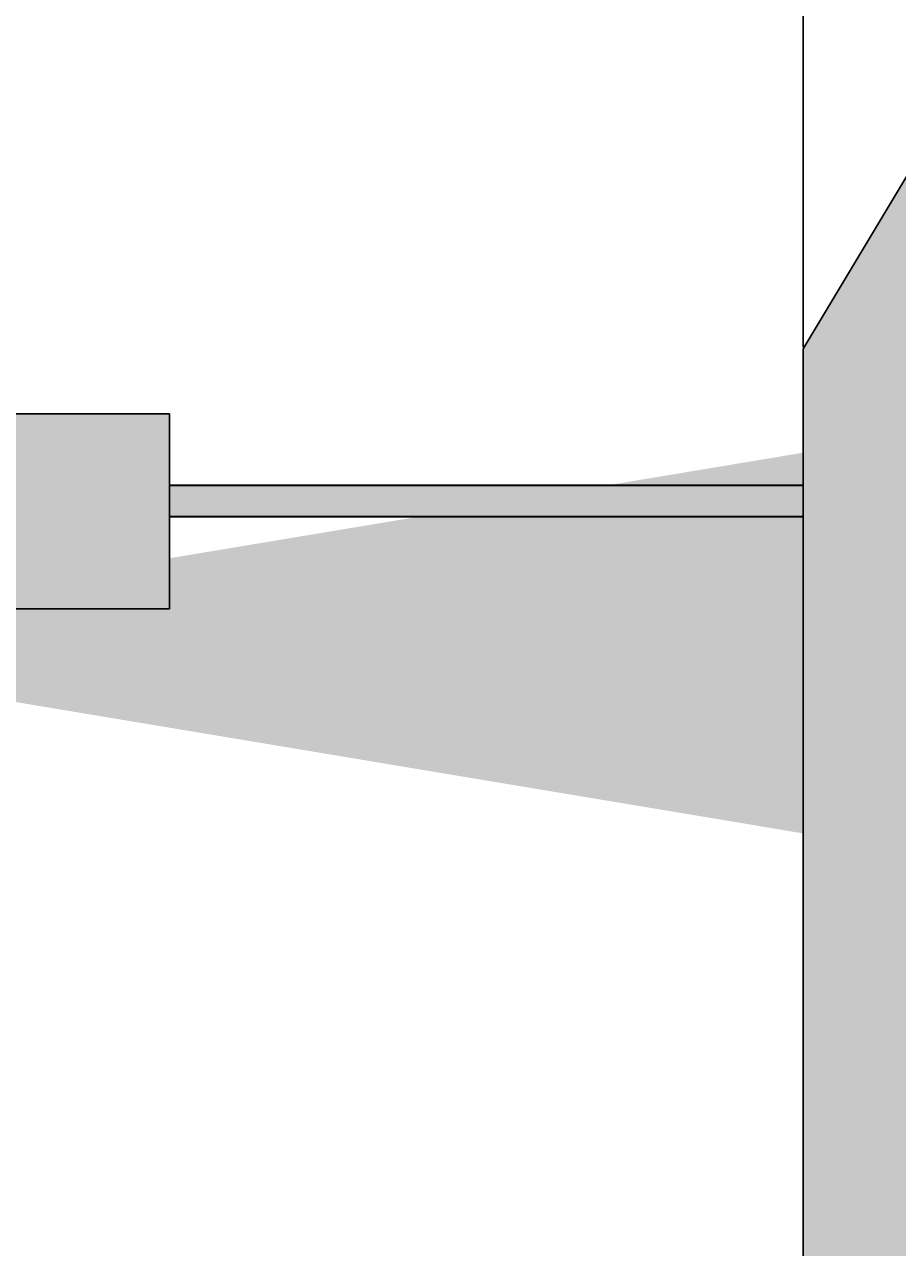
# Model space of a CAD drawing. Units: millimetres. Extents: x -22994 to 29398, y -19990 to 20176.
# Tile 24 of 135: x 71 to 99, y 99 to 138. Entities that reach past the tile are written whole.
import ezdxf

# ---------------------------------------------------------------- set-up
doc = ezdxf.new("R2010")
doc.units = ezdxf.units.MM
doc.header["$MEASUREMENT"] = 0
for name, color, linetype, lineweight in [('M-DIMS', 2, 'Continuous', 18), ('M-EQPM', 7, 'Continuous', 25), ('M-EQPM-PATT', 7, 'Continuous', 18), ('M-PIPE', 7, 'Continuous', 35)]:
    doc.layers.add(name, color=color, linetype=linetype, lineweight=lineweight)
doc.styles.get("Standard").update_dxf_attribs({"font": 'arial.ttf'})
doc.dimstyles.get("Standard").update_dxf_attribs({"dimtxt": 0.18, "dimasz": 10000, "dimexe": 0.18, "dimexo": 0.0625, "dimgap": 0.09, "dimtad": 0, "dimtih": 1, "dimtoh": 1, "dimdec": 0, "dimzin": 0, "dimdsep": 46, "dimtxsty": 'Standard', "dimcen": 0.09, "dimadec": 0, "dimazin": 0, "dimtfac": 1, "dimtdec": 0, "dimtofl": 0, "dimtmove": 0, "dimatfit": 3, "dimfxl": 1, "dimtolj": 1, "dimtzin": 0, "dimlwd": 30, "dimarcsym": 0})

# ---------------------------------------------------------------- blocks, each defined once
blk = doc.blocks.new('*D2')
at = {"layer": 'Defpoints', "color": 0, "transparency": 16777216}
for p in [(6.677, 10.271), (290.852, 10.271), (290.852, -5.079)]:
    blk.add_point(p, dxfattribs=at)
at = {"layer": 'M-DIMS', "color": 0, "lineweight": -2, "transparency": 16777216}
for p, q in [((6.677, 10.209), (6.677, -5.259)), ((290.852, 10.209), (290.852, -5.259))]:
    blk.add_line(p, q, dxfattribs=at)
at = {"layer": 'M-DIMS', "color": 0, "lineweight": 30, "transparency": 16777216}
for p, q in [((-9993.323, -5.079), (-19993.323, -5.079)), ((10290.852, -5.079), (20290.852, -5.079))]:
    blk.add_line(p, q, dxfattribs=at)
at = {"layer": 'M-DIMS', "color": 0, "transparency": 16777216}
for points in [[(-9993.323, 1661.588), (-9993.323, -1671.745), (6.677, -5.079)], [(10290.852, 1661.588), (10290.852, -1671.745), (290.852, -5.079)]]:
    blk.add_solid(points, dxfattribs=at)
at = {"layer": 'M-DIMS', "color": 0, "transparency": 16777216, "insert": (148.765, -5.079), "char_height": 0.18, "attachment_point": 5}
blk.add_mtext('\\A1;284.2', dxfattribs=at)
blk = doc.blocks.new('*D3')
at = {"layer": 'Defpoints', "color": 0, "transparency": 16777216}
for p in [(110.265, 204.165), (110.265, 176.366), (95.833, 127.967)]:
    blk.add_point(p, dxfattribs=at)
at = {"layer": 'M-DIMS', "color": 0, "lineweight": -2, "transparency": 16777216}
for p, q in [((95.833, 128.03), (95.833, 204.345)), ((110.265, 176.429), (110.265, 204.345))]:
    blk.add_line(p, q, dxfattribs=at)
at = {"layer": 'M-DIMS', "color": 0, "lineweight": 30, "transparency": 16777216}
for p, q in [((-9904.167, 204.165), (-19904.167, 204.165)), ((10110.265, 204.165), (20110.265, 204.165))]:
    blk.add_line(p, q, dxfattribs=at)
at = {"layer": 'M-DIMS', "color": 0, "transparency": 16777216}
for points in [[(-9904.167, 1870.832), (-9904.167, -1462.501), (95.833, 204.165)], [(10110.265, 1870.832), (10110.265, -1462.501), (110.265, 204.165)]]:
    blk.add_solid(points, dxfattribs=at)
at = {"layer": 'M-DIMS', "color": 0, "transparency": 16777216, "insert": (103.049, 204.165), "char_height": 0.18, "attachment_point": 5}
blk.add_mtext('\\A1;14.432', dxfattribs=at)
blk = doc.blocks.new('*D4')
at = {"layer": 'Defpoints', "color": 0, "transparency": 16777216}
for p in [(116.265, 204.165), (110.265, 176.366), (116.265, 176.366)]:
    blk.add_point(p, dxfattribs=at)
at = {"layer": 'M-DIMS', "color": 0, "lineweight": -2, "transparency": 16777216}
for p, q in [((110.265, 176.429), (110.265, 204.345)), ((116.265, 176.429), (116.265, 204.345))]:
    blk.add_line(p, q, dxfattribs=at)
at = {"layer": 'M-DIMS', "color": 0, "lineweight": 30, "transparency": 16777216}
for p, q in [((-9889.735, 204.165), (-19889.735, 204.165)), ((10116.265, 204.165), (20116.265, 204.165))]:
    blk.add_line(p, q, dxfattribs=at)
at = {"layer": 'M-DIMS', "color": 0, "transparency": 16777216}
for points in [[(-9889.735, 1870.832), (-9889.735, -1462.501), (110.265, 204.165)], [(10116.265, 1870.832), (10116.265, -1462.501), (116.265, 204.165)]]:
    blk.add_solid(points, dxfattribs=at)
at = {"layer": 'M-DIMS', "color": 0, "transparency": 16777216, "insert": (113.265, 204.165), "char_height": 0.18, "attachment_point": 5}
blk.add_mtext('\\A1;6', dxfattribs=at)
blk = doc.blocks.new('*D5')
at = {"layer": 'Defpoints', "color": 0, "transparency": 16777216}
for p in [(181.265, 204.165), (116.265, 176.366), (181.265, 176.366)]:
    blk.add_point(p, dxfattribs=at)
at = {"layer": 'M-DIMS', "color": 0, "lineweight": -2, "transparency": 16777216}
for p, q in [((116.265, 176.429), (116.265, 204.345)), ((181.265, 176.429), (181.265, 204.345))]:
    blk.add_line(p, q, dxfattribs=at)
at = {"layer": 'M-DIMS', "color": 0, "lineweight": 30, "transparency": 16777216}
for p, q in [((-9883.735, 204.165), (-19883.735, 204.165)), ((10181.265, 204.165), (20181.265, 204.165))]:
    blk.add_line(p, q, dxfattribs=at)
at = {"layer": 'M-DIMS', "color": 0, "transparency": 16777216}
for points in [[(-9883.735, 1870.832), (-9883.735, -1462.501), (116.265, 204.165)], [(10181.265, 1870.832), (10181.265, -1462.501), (181.265, 204.165)]]:
    blk.add_solid(points, dxfattribs=at)
at = {"layer": 'M-DIMS', "color": 0, "transparency": 16777216, "insert": (148.765, 204.165), "char_height": 0.18, "attachment_point": 5}
blk.add_mtext('\\A1;65', dxfattribs=at)
blk = doc.blocks.new('*D6')
at = {"layer": 'Defpoints', "color": 0, "transparency": 16777216}
for p in [(187.265, 204.165), (181.265, 176.366), (187.265, 176.366)]:
    blk.add_point(p, dxfattribs=at)
at = {"layer": 'M-DIMS', "color": 0, "lineweight": -2, "transparency": 16777216}
for p, q in [((181.265, 176.429), (181.265, 204.345)), ((187.265, 176.429), (187.265, 204.345))]:
    blk.add_line(p, q, dxfattribs=at)
at = {"layer": 'M-DIMS', "color": 0, "lineweight": 30, "transparency": 16777216}
for p, q in [((-9818.735, 204.165), (-19818.735, 204.165)), ((10187.265, 204.165), (20187.265, 204.165))]:
    blk.add_line(p, q, dxfattribs=at)
at = {"layer": 'M-DIMS', "color": 0, "transparency": 16777216}
for points in [[(-9818.735, 1870.832), (-9818.735, -1462.501), (181.265, 204.165)], [(10187.265, 1870.832), (10187.265, -1462.501), (187.265, 204.165)]]:
    blk.add_solid(points, dxfattribs=at)
at = {"layer": 'M-DIMS', "color": 0, "transparency": 16777216, "insert": (184.265, 204.165), "char_height": 0.18, "attachment_point": 5}
blk.add_mtext('\\A1;6', dxfattribs=at)
blk = doc.blocks.new('*D7')
at = {"layer": 'Defpoints', "color": 0, "transparency": 16777216}
for p in [(201.697, 204.165), (187.265, 176.366), (201.697, 127.967)]:
    blk.add_point(p, dxfattribs=at)
at = {"layer": 'M-DIMS', "color": 0, "lineweight": -2, "transparency": 16777216}
for p, q in [((187.265, 176.429), (187.265, 204.345)), ((201.697, 128.03), (201.697, 204.345))]:
    blk.add_line(p, q, dxfattribs=at)
at = {"layer": 'M-DIMS', "color": 0, "lineweight": 30, "transparency": 16777216}
for p, q in [((-9812.735, 204.165), (-19812.735, 204.165)), ((10201.697, 204.165), (20201.697, 204.165))]:
    blk.add_line(p, q, dxfattribs=at)
at = {"layer": 'M-DIMS', "color": 0, "transparency": 16777216}
for points in [[(-9812.735, 1870.832), (-9812.735, -1462.501), (187.265, 204.165)], [(10201.697, 1870.832), (10201.697, -1462.501), (201.697, 204.165)]]:
    blk.add_solid(points, dxfattribs=at)
at = {"layer": 'M-DIMS', "color": 0, "transparency": 16777216, "insert": (194.481, 204.165), "char_height": 0.18, "attachment_point": 5}
blk.add_mtext('\\A1;14.432', dxfattribs=at)
blk = doc.blocks.new('*D8')
at = {"layer": 'Defpoints', "color": 0, "transparency": 16777216}
for p in [(227.648, 204.165), (227.648, 146.73), (201.697, 127.967)]:
    blk.add_point(p, dxfattribs=at)
at = {"layer": 'M-DIMS', "color": 0, "lineweight": -2, "transparency": 16777216}
for p, q in [((201.697, 128.03), (201.697, 204.345)), ((227.648, 146.792), (227.648, 204.345))]:
    blk.add_line(p, q, dxfattribs=at)
at = {"layer": 'M-DIMS', "color": 0, "lineweight": 30, "transparency": 16777216}
for p, q in [((-9798.303, 204.165), (-19798.303, 204.165)), ((10227.648, 204.165), (20227.648, 204.165))]:
    blk.add_line(p, q, dxfattribs=at)
at = {"layer": 'M-DIMS', "color": 0, "transparency": 16777216}
for points in [[(-9798.303, 1870.832), (-9798.303, -1462.501), (201.697, 204.165)], [(10227.648, 1870.832), (10227.648, -1462.501), (227.648, 204.165)]]:
    blk.add_solid(points, dxfattribs=at)
at = {"layer": 'M-DIMS', "color": 0, "transparency": 16777216, "insert": (214.673, 204.165), "char_height": 0.18, "attachment_point": 5}
blk.add_mtext('\\A1;25.95', dxfattribs=at)
blk = doc.blocks.new('*D9')
at = {"layer": 'Defpoints', "color": 0, "transparency": 16777216}
for p in [(187.265, 176.366), (306.202, 176.366), (290.852, 10.271)]:
    blk.add_point(p, dxfattribs=at)
at = {"layer": 'M-DIMS', "color": 0, "lineweight": 30, "transparency": 16777216}
for p, q in [((306.202, 10176.366), (306.202, 20176.366)), ((306.202, -9989.729), (306.202, -19989.729))]:
    blk.add_line(p, q, dxfattribs=at)
at = {"layer": 'M-DIMS', "color": 0, "lineweight": -2, "transparency": 16777216}
for p, q in [((187.327, 176.366), (306.382, 176.366)), ((290.915, 10.271), (306.382, 10.271))]:
    blk.add_line(p, q, dxfattribs=at)
at = {"layer": 'M-DIMS', "color": 0, "transparency": 16777216}
for points in [[(-1360.465, 10176.366), (1972.869, 10176.366), (306.202, 176.366)], [(-1360.465, -9989.729), (1972.869, -9989.729), (306.202, 10.271)]]:
    blk.add_solid(points, dxfattribs=at)
at = {"layer": 'M-DIMS', "color": 0, "transparency": 16777216, "insert": (306.202, 93.319), "char_height": 0.18, "attachment_point": 5}
blk.add_mtext('\\A1;166.1', dxfattribs=at)
blk = doc.blocks.new('*D10')
at = {"layer": 'Defpoints', "color": 0, "transparency": 16777216}
for p in [(125.65, 136.071), (133.346, 136.071), (133.346, -5.079)]:
    blk.add_point(p, dxfattribs=at)
at = {"layer": 'M-DIMS', "color": 0, "lineweight": -2, "transparency": 16777216}
for p, q in [((125.65, 136.009), (125.65, -5.259)), ((133.346, 136.009), (133.346, -5.259))]:
    blk.add_line(p, q, dxfattribs=at)
at = {"layer": 'M-DIMS', "color": 0, "lineweight": 30, "transparency": 16777216}
for p, q in [((-9874.35, -5.079), (-19874.35, -5.079)), ((10133.346, -5.079), (20133.346, -5.079))]:
    blk.add_line(p, q, dxfattribs=at)
at = {"layer": 'M-DIMS', "color": 0, "transparency": 16777216}
for points in [[(-9874.35, 1661.588), (-9874.35, -1671.745), (125.65, -5.079)], [(10133.346, 1661.588), (10133.346, -1671.745), (133.346, -5.079)]]:
    blk.add_solid(points, dxfattribs=at)
at = {"layer": 'M-DIMS', "color": 0, "transparency": 16777216, "insert": (129.498, -5.079), "char_height": 0.18, "attachment_point": 5}
blk.add_mtext('\\A1;7.696', dxfattribs=at)
blk = doc.blocks.new('*D11')
at = {"layer": 'Defpoints', "color": 0, "transparency": 16777216}
for p in [(133.346, 136.071), (135.65, 136.071), (135.65, -5.079)]:
    blk.add_point(p, dxfattribs=at)
at = {"layer": 'M-DIMS', "color": 0, "lineweight": -2, "transparency": 16777216}
for p, q in [((133.346, 136.009), (133.346, -5.259)), ((135.65, 136.009), (135.65, -5.259))]:
    blk.add_line(p, q, dxfattribs=at)
at = {"layer": 'M-DIMS', "color": 0, "lineweight": 30, "transparency": 16777216}
for p, q in [((-9866.654, -5.079), (-19866.654, -5.079)), ((10135.65, -5.079), (20135.65, -5.079))]:
    blk.add_line(p, q, dxfattribs=at)
at = {"layer": 'M-DIMS', "color": 0, "transparency": 16777216}
for points in [[(-9866.654, 1661.588), (-9866.654, -1671.745), (133.346, -5.079)], [(10135.65, 1661.588), (10135.65, -1671.745), (135.65, -5.079)]]:
    blk.add_solid(points, dxfattribs=at)
at = {"layer": 'M-DIMS', "color": 0, "transparency": 16777216, "insert": (134.498, -5.079), "char_height": 0.18, "attachment_point": 5}
blk.add_mtext('\\A1;2.304', dxfattribs=at)
blk = doc.blocks.new('*D12')
at = {"layer": 'Defpoints', "color": 0, "transparency": 16777216}
for p in [(135.65, 136.071), (145.65, 136.071), (145.65, -5.079)]:
    blk.add_point(p, dxfattribs=at)
at = {"layer": 'M-DIMS', "color": 0, "lineweight": -2, "transparency": 16777216}
for p, q in [((135.65, 136.009), (135.65, -5.259)), ((145.65, 136.009), (145.65, -5.259))]:
    blk.add_line(p, q, dxfattribs=at)
at = {"layer": 'M-DIMS', "color": 0, "lineweight": 30, "transparency": 16777216}
for p, q in [((-9864.35, -5.079), (-19864.35, -5.079)), ((10145.65, -5.079), (20145.65, -5.079))]:
    blk.add_line(p, q, dxfattribs=at)
at = {"layer": 'M-DIMS', "color": 0, "transparency": 16777216}
for points in [[(-9864.35, 1661.588), (-9864.35, -1671.745), (135.65, -5.079)], [(10145.65, 1661.588), (10145.65, -1671.745), (145.65, -5.079)]]:
    blk.add_solid(points, dxfattribs=at)
at = {"layer": 'M-DIMS', "color": 0, "transparency": 16777216, "insert": (140.65, -5.079), "char_height": 0.18, "attachment_point": 5}
blk.add_mtext('\\A1;10', dxfattribs=at)
blk = doc.blocks.new('*D13')
at = {"layer": 'Defpoints', "color": 0, "transparency": 16777216}
for p in [(145.65, 136.071), (155.65, 136.071), (155.65, -5.079)]:
    blk.add_point(p, dxfattribs=at)
at = {"layer": 'M-DIMS', "color": 0, "lineweight": -2, "transparency": 16777216}
for p, q in [((145.65, 136.009), (145.65, -5.259)), ((155.65, 136.009), (155.65, -5.259))]:
    blk.add_line(p, q, dxfattribs=at)
at = {"layer": 'M-DIMS', "color": 0, "lineweight": 30, "transparency": 16777216}
for p, q in [((-9854.35, -5.079), (-19854.35, -5.079)), ((10155.65, -5.079), (20155.65, -5.079))]:
    blk.add_line(p, q, dxfattribs=at)
at = {"layer": 'M-DIMS', "color": 0, "transparency": 16777216}
for points in [[(-9854.35, 1661.588), (-9854.35, -1671.745), (145.65, -5.079)], [(10155.65, 1661.588), (10155.65, -1671.745), (155.65, -5.079)]]:
    blk.add_solid(points, dxfattribs=at)
at = {"layer": 'M-DIMS', "color": 0, "transparency": 16777216, "insert": (150.65, -5.079), "char_height": 0.18, "attachment_point": 5}
blk.add_mtext('\\A1;10', dxfattribs=at)
blk = doc.blocks.new('*D14')
at = {"layer": 'Defpoints', "color": 0, "transparency": 16777216}
for p in [(155.65, 136.071), (165.65, 136.071), (165.65, -5.079)]:
    blk.add_point(p, dxfattribs=at)
at = {"layer": 'M-DIMS', "color": 0, "lineweight": -2, "transparency": 16777216}
for p, q in [((155.65, 136.009), (155.65, -5.259)), ((165.65, 136.009), (165.65, -5.259))]:
    blk.add_line(p, q, dxfattribs=at)
at = {"layer": 'M-DIMS', "color": 0, "lineweight": 30, "transparency": 16777216}
for p, q in [((-9844.35, -5.079), (-19844.35, -5.079)), ((10165.65, -5.079), (20165.65, -5.079))]:
    blk.add_line(p, q, dxfattribs=at)
at = {"layer": 'M-DIMS', "color": 0, "transparency": 16777216}
for points in [[(-9844.35, 1661.588), (-9844.35, -1671.745), (155.65, -5.079)], [(10165.65, 1661.588), (10165.65, -1671.745), (165.65, -5.079)]]:
    blk.add_solid(points, dxfattribs=at)
at = {"layer": 'M-DIMS', "color": 0, "transparency": 16777216, "insert": (160.65, -5.079), "char_height": 0.18, "attachment_point": 5}
blk.add_mtext('\\A1;10', dxfattribs=at)
blk = doc.blocks.new('*D15')
at = {"layer": 'Defpoints', "color": 0, "transparency": 16777216}
for p in [(173.346, 154.788), (173.346, 136.071), (306.202, 136.071)]:
    blk.add_point(p, dxfattribs=at)
at = {"layer": 'M-DIMS', "color": 0, "lineweight": 30, "transparency": 16777216}
for p, q in [((306.202, 10154.788), (306.202, 20154.788)), ((306.202, -9863.929), (306.202, -19863.929))]:
    blk.add_line(p, q, dxfattribs=at)
at = {"layer": 'M-DIMS', "color": 0, "lineweight": -2, "transparency": 16777216}
for p, q in [((173.408, 154.788), (306.382, 154.788)), ((173.408, 136.071), (306.382, 136.071))]:
    blk.add_line(p, q, dxfattribs=at)
at = {"layer": 'M-DIMS', "color": 0, "transparency": 16777216}
for points in [[(-1360.465, 10154.788), (1972.869, 10154.788), (306.202, 154.788)], [(-1360.465, -9863.929), (1972.869, -9863.929), (306.202, 136.071)]]:
    blk.add_solid(points, dxfattribs=at)
at = {"layer": 'M-DIMS', "color": 0, "transparency": 16777216, "insert": (306.202, 145.43), "char_height": 0.18, "attachment_point": 5}
blk.add_mtext('\\A1;18.717', dxfattribs=at)
blk = doc.blocks.new('*D16')
at = {"layer": 'Defpoints', "color": 0, "transparency": 16777216}
for p in [(120.17, 204.165), (110.466, 48.035), (120.17, 48.035)]:
    blk.add_point(p, dxfattribs=at)
at = {"layer": 'M-DIMS', "color": 0, "lineweight": -2, "transparency": 16777216}
for p, q in [((110.466, 48.097), (110.466, 204.345)), ((120.17, 48.097), (120.17, 204.345))]:
    blk.add_line(p, q, dxfattribs=at)
at = {"layer": 'M-DIMS', "color": 0, "lineweight": 30, "transparency": 16777216}
for p, q in [((-9889.534, 204.165), (-19889.534, 204.165)), ((10120.17, 204.165), (20120.17, 204.165))]:
    blk.add_line(p, q, dxfattribs=at)
at = {"layer": 'M-DIMS', "color": 0, "transparency": 16777216}
for points in [[(-9889.534, 1870.832), (-9889.534, -1462.501), (110.466, 204.165)], [(10120.17, 1870.832), (10120.17, -1462.501), (120.17, 204.165)]]:
    blk.add_solid(points, dxfattribs=at)
at = {"layer": 'M-DIMS', "color": 0, "transparency": 16777216, "insert": (115.318, 204.165), "char_height": 0.18, "attachment_point": 5}
blk.add_mtext('\\A1;9.704', dxfattribs=at)
blk = doc.blocks.new('*D17')
at = {"layer": 'Defpoints', "color": 0, "transparency": 16777216}
for p in [(126.17, 204.165), (120.17, 48.035), (126.17, 48.035)]:
    blk.add_point(p, dxfattribs=at)
at = {"layer": 'M-DIMS', "color": 0, "lineweight": -2, "transparency": 16777216}
for p, q in [((120.17, 48.097), (120.17, 204.345)), ((126.17, 48.097), (126.17, 204.345))]:
    blk.add_line(p, q, dxfattribs=at)
at = {"layer": 'M-DIMS', "color": 0, "lineweight": 30, "transparency": 16777216}
for p, q in [((-9879.83, 204.165), (-19879.83, 204.165)), ((10126.17, 204.165), (20126.17, 204.165))]:
    blk.add_line(p, q, dxfattribs=at)
at = {"layer": 'M-DIMS', "color": 0, "transparency": 16777216}
for points in [[(-9879.83, 1870.832), (-9879.83, -1462.501), (120.17, 204.165)], [(10126.17, 1870.832), (10126.17, -1462.501), (126.17, 204.165)]]:
    blk.add_solid(points, dxfattribs=at)
at = {"layer": 'M-DIMS', "color": 0, "transparency": 16777216, "insert": (123.17, 204.165), "char_height": 0.18, "attachment_point": 5}
blk.add_mtext('\\A1;6', dxfattribs=at)
blk = doc.blocks.new('*D18')
at = {"layer": 'Defpoints', "color": 0, "transparency": 16777216}
for p in [(132.17, 204.165), (126.17, 48.035), (132.17, 48.035)]:
    blk.add_point(p, dxfattribs=at)
at = {"layer": 'M-DIMS', "color": 0, "lineweight": -2, "transparency": 16777216}
for p, q in [((126.17, 48.097), (126.17, 204.345)), ((132.17, 48.097), (132.17, 204.345))]:
    blk.add_line(p, q, dxfattribs=at)
at = {"layer": 'M-DIMS', "color": 0, "lineweight": 30, "transparency": 16777216}
for p, q in [((-9873.83, 204.165), (-19873.83, 204.165)), ((10132.17, 204.165), (20132.17, 204.165))]:
    blk.add_line(p, q, dxfattribs=at)
at = {"layer": 'M-DIMS', "color": 0, "transparency": 16777216}
for points in [[(-9873.83, 1870.832), (-9873.83, -1462.501), (126.17, 204.165)], [(10132.17, 1870.832), (10132.17, -1462.501), (132.17, 204.165)]]:
    blk.add_solid(points, dxfattribs=at)
at = {"layer": 'M-DIMS', "color": 0, "transparency": 16777216, "insert": (129.17, 204.165), "char_height": 0.18, "attachment_point": 5}
blk.add_mtext('\\A1;6', dxfattribs=at)
blk = doc.blocks.new('*D19')
at = {"layer": 'Defpoints', "color": 0, "transparency": 16777216}
for p in [(138.17, 204.165), (132.17, 48.035), (138.17, 48.035)]:
    blk.add_point(p, dxfattribs=at)
at = {"layer": 'M-DIMS', "color": 0, "lineweight": -2, "transparency": 16777216}
for p, q in [((132.17, 48.097), (132.17, 204.345)), ((138.17, 48.097), (138.17, 204.345))]:
    blk.add_line(p, q, dxfattribs=at)
at = {"layer": 'M-DIMS', "color": 0, "lineweight": 30, "transparency": 16777216}
for p, q in [((-9867.83, 204.165), (-19867.83, 204.165)), ((10138.17, 204.165), (20138.17, 204.165))]:
    blk.add_line(p, q, dxfattribs=at)
at = {"layer": 'M-DIMS', "color": 0, "transparency": 16777216}
for points in [[(-9867.83, 1870.832), (-9867.83, -1462.501), (132.17, 204.165)], [(10138.17, 1870.832), (10138.17, -1462.501), (138.17, 204.165)]]:
    blk.add_solid(points, dxfattribs=at)
at = {"layer": 'M-DIMS', "color": 0, "transparency": 16777216, "insert": (135.17, 204.165), "char_height": 0.18, "attachment_point": 5}
blk.add_mtext('\\A1;6', dxfattribs=at)
blk = doc.blocks.new('*D20')
at = {"layer": 'Defpoints', "color": 0, "transparency": 16777216}
for p in [(144.17, 204.165), (138.17, 48.035), (144.17, 48.035)]:
    blk.add_point(p, dxfattribs=at)
at = {"layer": 'M-DIMS', "color": 0, "lineweight": -2, "transparency": 16777216}
for p, q in [((138.17, 48.097), (138.17, 204.345)), ((144.17, 48.097), (144.17, 204.345))]:
    blk.add_line(p, q, dxfattribs=at)
at = {"layer": 'M-DIMS', "color": 0, "lineweight": 30, "transparency": 16777216}
for p, q in [((-9861.83, 204.165), (-19861.83, 204.165)), ((10144.17, 204.165), (20144.17, 204.165))]:
    blk.add_line(p, q, dxfattribs=at)
at = {"layer": 'M-DIMS', "color": 0, "transparency": 16777216}
for points in [[(-9861.83, 1870.832), (-9861.83, -1462.501), (138.17, 204.165)], [(10144.17, 1870.832), (10144.17, -1462.501), (144.17, 204.165)]]:
    blk.add_solid(points, dxfattribs=at)
at = {"layer": 'M-DIMS', "color": 0, "transparency": 16777216, "insert": (141.17, 204.165), "char_height": 0.18, "attachment_point": 5}
blk.add_mtext('\\A1;6', dxfattribs=at)
blk = doc.blocks.new('*D21')
at = {"layer": 'Defpoints', "color": 0, "transparency": 16777216}
for p in [(149.116, 204.165), (144.17, 48.035), (149.116, 48.035)]:
    blk.add_point(p, dxfattribs=at)
at = {"layer": 'M-DIMS', "color": 0, "lineweight": -2, "transparency": 16777216}
for p, q in [((144.17, 48.097), (144.17, 204.345)), ((149.116, 48.097), (149.116, 204.345))]:
    blk.add_line(p, q, dxfattribs=at)
at = {"layer": 'M-DIMS', "color": 0, "lineweight": 30, "transparency": 16777216}
for p, q in [((-9855.83, 204.165), (-19855.83, 204.165)), ((10149.116, 204.165), (20149.116, 204.165))]:
    blk.add_line(p, q, dxfattribs=at)
at = {"layer": 'M-DIMS', "color": 0, "transparency": 16777216}
for points in [[(-9855.83, 1870.832), (-9855.83, -1462.501), (144.17, 204.165)], [(10149.116, 1870.832), (10149.116, -1462.501), (149.116, 204.165)]]:
    blk.add_solid(points, dxfattribs=at)
at = {"layer": 'M-DIMS', "color": 0, "transparency": 16777216, "insert": (146.643, 204.165), "char_height": 0.18, "attachment_point": 5}
blk.add_mtext('\\A1;4.945', dxfattribs=at)
blk = doc.blocks.new('*D22')
at = {"layer": 'Defpoints', "color": 0, "transparency": 16777216}
for p in [(149.116, 30.99), (155.116, 30.99), (155.116, -5.079)]:
    blk.add_point(p, dxfattribs=at)
at = {"layer": 'M-DIMS', "color": 0, "lineweight": -2, "transparency": 16777216}
for p, q in [((149.116, 30.927), (149.116, -5.259)), ((155.116, 30.927), (155.116, -5.259))]:
    blk.add_line(p, q, dxfattribs=at)
at = {"layer": 'M-DIMS', "color": 0, "lineweight": 30, "transparency": 16777216}
for p, q in [((-9850.884, -5.079), (-19850.884, -5.079)), ((10155.116, -5.079), (20155.116, -5.079))]:
    blk.add_line(p, q, dxfattribs=at)
at = {"layer": 'M-DIMS', "color": 0, "transparency": 16777216}
for points in [[(-9850.884, 1661.588), (-9850.884, -1671.745), (149.116, -5.079)], [(10155.116, 1661.588), (10155.116, -1671.745), (155.116, -5.079)]]:
    blk.add_solid(points, dxfattribs=at)
at = {"layer": 'M-DIMS', "color": 0, "transparency": 16777216, "insert": (152.116, -5.079), "char_height": 0.18, "attachment_point": 5}
blk.add_mtext('\\A1;6', dxfattribs=at)
blk = doc.blocks.new('*D23')
at = {"layer": 'Defpoints', "color": 0, "transparency": 16777216}
for p in [(155.116, 30.99), (161.116, 30.99), (161.116, -5.079)]:
    blk.add_point(p, dxfattribs=at)
at = {"layer": 'M-DIMS', "color": 0, "lineweight": -2, "transparency": 16777216}
for p, q in [((155.116, 30.927), (155.116, -5.259)), ((161.116, 30.927), (161.116, -5.259))]:
    blk.add_line(p, q, dxfattribs=at)
at = {"layer": 'M-DIMS', "color": 0, "lineweight": 30, "transparency": 16777216}
for p, q in [((-9844.884, -5.079), (-19844.884, -5.079)), ((10161.116, -5.079), (20161.116, -5.079))]:
    blk.add_line(p, q, dxfattribs=at)
at = {"layer": 'M-DIMS', "color": 0, "transparency": 16777216}
for points in [[(-9844.884, 1661.588), (-9844.884, -1671.745), (155.116, -5.079)], [(10161.116, 1661.588), (10161.116, -1671.745), (161.116, -5.079)]]:
    blk.add_solid(points, dxfattribs=at)
at = {"layer": 'M-DIMS', "color": 0, "transparency": 16777216, "insert": (158.116, -5.079), "char_height": 0.18, "attachment_point": 5}
blk.add_mtext('\\A1;6', dxfattribs=at)
blk = doc.blocks.new('*D24')
at = {"layer": 'Defpoints', "color": 0, "transparency": 16777216}
for p in [(161.116, 30.99), (166.439, 30.99), (166.439, -5.079)]:
    blk.add_point(p, dxfattribs=at)
at = {"layer": 'M-DIMS', "color": 0, "lineweight": -2, "transparency": 16777216}
for p, q in [((161.116, 30.927), (161.116, -5.259)), ((166.439, 30.927), (166.439, -5.259))]:
    blk.add_line(p, q, dxfattribs=at)
at = {"layer": 'M-DIMS', "color": 0, "lineweight": 30, "transparency": 16777216}
for p, q in [((-9838.884, -5.079), (-19838.884, -5.079)), ((10166.439, -5.079), (20166.439, -5.079))]:
    blk.add_line(p, q, dxfattribs=at)
at = {"layer": 'M-DIMS', "color": 0, "transparency": 16777216}
for points in [[(-9838.884, 1661.588), (-9838.884, -1671.745), (161.116, -5.079)], [(10166.439, 1661.588), (10166.439, -1671.745), (166.439, -5.079)]]:
    blk.add_solid(points, dxfattribs=at)
at = {"layer": 'M-DIMS', "color": 0, "transparency": 16777216, "insert": (163.777, -5.079), "char_height": 0.18, "attachment_point": 5}
blk.add_mtext('\\A1;5.323', dxfattribs=at)
blk = doc.blocks.new('*D25')
at = {"layer": 'Defpoints', "color": 0, "transparency": 16777216}
for p in [(166.439, 30.99), (172.439, 30.99), (172.439, -5.079)]:
    blk.add_point(p, dxfattribs=at)
at = {"layer": 'M-DIMS', "color": 0, "lineweight": -2, "transparency": 16777216}
for p, q in [((166.439, 30.927), (166.439, -5.259)), ((172.439, 30.927), (172.439, -5.259))]:
    blk.add_line(p, q, dxfattribs=at)
at = {"layer": 'M-DIMS', "color": 0, "lineweight": 30, "transparency": 16777216}
for p, q in [((-9833.561, -5.079), (-19833.561, -5.079)), ((10172.439, -5.079), (20172.439, -5.079))]:
    blk.add_line(p, q, dxfattribs=at)
at = {"layer": 'M-DIMS', "color": 0, "transparency": 16777216}
for points in [[(-9833.561, 1661.588), (-9833.561, -1671.745), (166.439, -5.079)], [(10172.439, 1661.588), (10172.439, -1671.745), (172.439, -5.079)]]:
    blk.add_solid(points, dxfattribs=at)
at = {"layer": 'M-DIMS', "color": 0, "transparency": 16777216, "insert": (169.439, -5.079), "char_height": 0.18, "attachment_point": 5}
blk.add_mtext('\\A1;6', dxfattribs=at)
blk = doc.blocks.new('*D26')
at = {"layer": 'Defpoints', "color": 0, "transparency": 16777216}
for p in [(172.439, 30.99), (178.439, 30.99), (178.439, -5.079)]:
    blk.add_point(p, dxfattribs=at)
at = {"layer": 'M-DIMS', "color": 0, "lineweight": -2, "transparency": 16777216}
for p, q in [((172.439, 30.927), (172.439, -5.259)), ((178.439, 30.927), (178.439, -5.259))]:
    blk.add_line(p, q, dxfattribs=at)
at = {"layer": 'M-DIMS', "color": 0, "lineweight": 30, "transparency": 16777216}
for p, q in [((-9827.561, -5.079), (-19827.561, -5.079)), ((10178.439, -5.079), (20178.439, -5.079))]:
    blk.add_line(p, q, dxfattribs=at)
at = {"layer": 'M-DIMS', "color": 0, "transparency": 16777216}
for points in [[(-9827.561, 1661.588), (-9827.561, -1671.745), (172.439, -5.079)], [(10178.439, 1661.588), (10178.439, -1671.745), (178.439, -5.079)]]:
    blk.add_solid(points, dxfattribs=at)
at = {"layer": 'M-DIMS', "color": 0, "transparency": 16777216, "insert": (175.439, -5.079), "char_height": 0.18, "attachment_point": 5}
blk.add_mtext('\\A1;6', dxfattribs=at)
blk = doc.blocks.new('*D27')
at = {"layer": 'Defpoints', "color": 0, "transparency": 16777216}
for p in [(178.439, 30.99), (188.117, 30.99), (188.117, -5.079)]:
    blk.add_point(p, dxfattribs=at)
at = {"layer": 'M-DIMS', "color": 0, "lineweight": -2, "transparency": 16777216}
for p, q in [((178.439, 30.927), (178.439, -5.259)), ((188.117, 30.927), (188.117, -5.259))]:
    blk.add_line(p, q, dxfattribs=at)
at = {"layer": 'M-DIMS', "color": 0, "lineweight": 30, "transparency": 16777216}
for p, q in [((-9821.561, -5.079), (-19821.561, -5.079)), ((10188.117, -5.079), (20188.117, -5.079))]:
    blk.add_line(p, q, dxfattribs=at)
at = {"layer": 'M-DIMS', "color": 0, "transparency": 16777216}
for points in [[(-9821.561, 1661.588), (-9821.561, -1671.745), (178.439, -5.079)], [(10188.117, 1661.588), (10188.117, -1671.745), (188.117, -5.079)]]:
    blk.add_solid(points, dxfattribs=at)
at = {"layer": 'M-DIMS', "color": 0, "transparency": 16777216, "insert": (183.278, -5.079), "char_height": 0.18, "attachment_point": 5}
blk.add_mtext('\\A1;9.679', dxfattribs=at)
blk = doc.blocks.new('*D28')
at = {"layer": 'Defpoints', "color": 0, "transparency": 16777216}
for p in [(188.117, 48.035), (306.202, 48.035), (188.117, 30.99)]:
    blk.add_point(p, dxfattribs=at)
at = {"layer": 'M-DIMS', "color": 0, "lineweight": 30, "transparency": 16777216}
for p, q in [((306.202, 10048.035), (306.202, 20048.035)), ((306.202, -9969.01), (306.202, -19969.01))]:
    blk.add_line(p, q, dxfattribs=at)
at = {"layer": 'M-DIMS', "color": 0, "lineweight": -2, "transparency": 16777216}
for p, q in [((188.18, 48.035), (306.382, 48.035)), ((188.18, 30.99), (306.382, 30.99))]:
    blk.add_line(p, q, dxfattribs=at)
at = {"layer": 'M-DIMS', "color": 0, "transparency": 16777216}
for points in [[(-1360.465, 10048.035), (1972.869, 10048.035), (306.202, 48.035)], [(-1360.465, -9969.01), (1972.869, -9969.01), (306.202, 30.99)]]:
    blk.add_solid(points, dxfattribs=at)
at = {"layer": 'M-DIMS', "color": 0, "transparency": 16777216, "insert": (306.202, 39.512), "char_height": 0.18, "attachment_point": 5}
blk.add_mtext('\\A1;17.045', dxfattribs=at)
blk = doc.blocks.new('*D29')
at = {"layer": 'Defpoints', "color": 0, "transparency": 16777216}
for p in [(36.801, 80.045), (64.03, 80.045)]:
    blk.add_point(p, dxfattribs=at)
at = {"layer": 'M-DIMS', "color": 0, "lineweight": -2, "transparency": 16777216}
for p, q in [((50.325, 80.045), (50.505, 80.045)), ((50.415, 79.955), (50.415, 80.135))]:
    blk.add_line(p, q, dxfattribs=at)
at = {"layer": 'M-DIMS', "color": 0, "lineweight": 30, "transparency": 16777216}
blk.add_line((20064.03, 80.03), (10064.03, 80.038), dxfattribs=at)
at = {"layer": 'M-DIMS', "color": 0, "transparency": 16777216}
blk.add_solid([(10064.031, 1746.704), (10064.028, -1586.629), (64.03, 80.045)], dxfattribs=at)
at = {"layer": 'M-DIMS', "color": 0, "transparency": 16777216, "insert": (20064.521, 80.03), "char_height": 0.18, "attachment_point": 5}
blk.add_mtext('\\A1;∅27.23', dxfattribs=at)
blk = doc.blocks.new('*D36')
at = {"layer": 'Defpoints', "color": 0, "transparency": 16777216}
for p in [(46.39, 31.303), (46.387, 26.593)]:
    blk.add_point(p, dxfattribs=at)
at = {"layer": 'M-DIMS', "color": 0, "lineweight": 30, "transparency": 16777216}
for p, q in [((57.15, 20031.301), (51.77, 10031.302)), ((10057.15, 20031.301), (57.15, 20031.301))]:
    blk.add_line(p, q, dxfattribs=at)
at = {"layer": 'M-DIMS', "color": 0, "lineweight": -2, "transparency": 16777216}
for p, q in [((46.299, 28.948), (46.479, 28.948)), ((46.389, 28.858), (46.389, 29.038))]:
    blk.add_line(p, q, dxfattribs=at)
at = {"layer": 'M-DIMS', "color": 0, "transparency": 16777216}
blk.add_solid([(-1614.896, 10032.199), (1718.436, 10030.405), (46.39, 31.303)], dxfattribs=at)
at = {"layer": 'M-DIMS', "color": 0, "transparency": 16777216, "insert": (10057.554, 20031.301), "char_height": 0.18, "attachment_point": 5}
blk.add_mtext('\\A1;∅4.71', dxfattribs=at)
blk = doc.blocks.new('*D37')
at = {"layer": 'Defpoints', "color": 0, "transparency": 16777216}
for p in [(54.834, 118.615), (59.494, 118.614)]:
    blk.add_point(p, dxfattribs=at)
at = {"layer": 'M-DIMS', "color": 0, "lineweight": -2, "transparency": 16777216}
for p, q in [((57.164, 118.524), (57.164, 118.704)), ((57.074, 118.614), (57.254, 118.614))]:
    blk.add_line(p, q, dxfattribs=at)
at = {"layer": 'M-DIMS', "color": 0, "lineweight": 30, "transparency": 16777216}
blk.add_line((20059.493, 116.253), (10059.494, 117.434), dxfattribs=at)
at = {"layer": 'M-DIMS', "color": 0, "transparency": 16777216}
blk.add_solid([(10059.69, 1784.1), (10059.297, -1549.233), (59.494, 118.614)], dxfattribs=at)
at = {"layer": 'M-DIMS', "color": 0, "transparency": 16777216, "insert": (20059.985, 116.253), "char_height": 0.18, "attachment_point": 5}
blk.add_mtext('\\A1;∅4.659', dxfattribs=at)

msp = doc.modelspace()

# ---------------------------------------------------------------- hatches: boundary and pattern name
at = {"layer": 'M-EQPM-PATT'}
h = msp.add_hatch(color=256, dxfattribs=at)
h.set_gradient(color1=(205, 32, 39), color2=(205, 32, 39), tint=1)
h.paths.add_polyline_path([(116.2647, 150.3662), (116.2647, 170.3662), (116.2647, 176.3662), (110.2647, 176.3662), (110.2647, 152.0276), (95.8327, 127.967), (95.8327, 16.6063), (201.6967, 16.6063), (201.6967, 127.967), (187.2647, 152.0276), (187.2647, 176.3662), (181.2647, 176.3662), (181.2647, 170.3662), (181.2647, 150.3662), (195.6967, 126.3055), (195.6967, 22.6063), (101.8327, 22.6063), (101.8327, 126.3055)])
h.paths.add_polyline_path([(185.2208, 88.6347), (101.8327, 88.6347), (101.8327, 87.6347), (182.8066, 87.6347), (178.7313, 83.5594), (195.6967, 83.5594), (195.6967, 84.5594), (181.1455, 84.5594)], flags=17)
h.paths.add_polyline_path([(95.8327, 88.6347), (60.9779, 88.6347, -0.0228552), (61.7178, 87.6347), (95.8327, 87.6347)])
h.paths.add_polyline_path([(215.6212, 86.5189), (215.6212, 80.5999), (220.5095, 83.5594)])
h.paths.add_polyline_path([(215.6212, 84.5594), (201.6967, 84.5594), (201.6967, 83.5594), (215.6212, 83.5594)])
h.paths.add_polyline_path([(225.3978, 86.5189), (220.5095, 83.5594), (225.3978, 80.5999)])
h.paths.add_polyline_path([(231.6256, 84.5594), (225.3978, 84.5594), (225.3978, 83.5594), (231.6256, 83.5594)])
h = msp.add_hatch(color=256, dxfattribs=at)
h.set_gradient(color1=(242, 103, 34), color2=(242, 103, 34), tint=1, name='CYLINDER')
h.paths.add_polyline_path([(53.5912, 30.0354), (64.8905, 30.0354), (64.8905, 36.2325), (46.3887, 36.2325, 2.6954641)])
h.paths.add_polyline_path([(44.0337, 28.9485, -1), (48.7438, 28.9485, -1)], flags=16)
h.paths.add_polyline_path([(75.6657, 119.7012), (75.6657, 125.8983), (57.1639, 125.8983, 2.6954641), (64.3664, 119.7012)])
h.paths.add_polyline_path([(59.4936, 118.6143, -1), (54.8343, 118.6143, -1)], flags=16)
h = msp.add_hatch(color=256, dxfattribs=at)
h.set_gradient(color1=(34, 52, 110), color2=(41, 49, 137), tint=1, name='CYLINDER')
h.paths.add_polyline_path([(101.8327, 123.6277), (101.8327, 122.6277), (176.8123, 122.6277, -0.4142136), (178.3123, 121.1277), (178.3123, 119.1277, -0.4142136), (176.8123, 117.6277), (129.8123, 117.6277, 0.4142136), (128.3123, 116.1277), (128.3123, 114.1277, 0.4142136), (129.8123, 112.6277), (176.8123, 112.6277, -0.4142136), (178.3123, 111.1277), (178.3123, 109.1277, -0.4142136), (176.8123, 107.6277), (129.8123, 107.6277, 0.4142136), (128.3123, 106.1277), (128.3123, 104.1277, 0.4142136), (129.8123, 102.6277), (176.8123, 102.6277, -0.4142136), (178.3123, 101.1277), (178.3123, 99.1277, -0.4142136), (176.8123, 97.6277), (101.8327, 97.6277), (101.8327, 96.6277), (176.8123, 96.6277, 0.4142136), (179.3123, 99.1277), (179.3123, 101.1277, 0.4142136), (176.8123, 103.6277), (129.8123, 103.6277, -0.4142136), (129.3123, 104.1277), (129.3123, 106.1277, -0.4142136), (129.8123, 106.6277), (176.8123, 106.6277, 0.4142136), (179.3123, 109.1277), (179.3123, 111.1277, 0.4142136), (176.8123, 113.6277), (129.8123, 113.6277, -0.4142136), (129.3123, 114.1277), (129.3123, 116.1277, -0.4142136), (129.8123, 116.6277), (176.8123, 116.6277, 0.4142136), (179.3123, 119.1277), (179.3123, 121.1277, 0.4142136), (176.8123, 123.6277)])
h.paths.add_polyline_path([(75.6657, 123.6277), (75.6657, 122.6277), (95.8327, 122.6277), (95.8327, 123.6277)])
h.paths.add_polyline_path([(51.0853, 122.6277, -0.0439182), (51.8797, 123.6277), (38.9157, 123.6277), (38.9157, 122.6277)])
h.paths.add_polyline_path([(95.8327, 96.6277), (95.8327, 97.6277), (22.2694, 97.6277, 0.4142136), (20.7694, 96.1277), (20.7694, 89.8712, 0.4142136), (22.2694, 88.3712), (39.6435, 88.3712, -0.024152), (40.4967, 89.3712), (23.2694, 89.3712, -0.4142136), (21.7694, 90.8712), (21.7694, 95.1277, -0.4142136), (23.2694, 96.6277)])
h.paths.add_polyline_path([(137.7248, 106.4435), (168.6853, 106.4435), (168.6853, 114.6864), (137.7248, 114.6864)], flags=25)

# ---------------------------------------------------------------- linework, layer by layer
at = {"layer": 'M-EQPM'}
msp.add_lwpolyline([(110.2647, 176.3662), (110.2647, 152.0276), (95.8327, 127.967), (95.8327, 16.6063), (201.6967, 16.6063), (201.6967, 127.967), (187.2647, 152.0276), (187.2647, 176.3662)], close=True, dxfattribs=at)
msp.add_lwpolyline([(57.1639, 125.8983), (75.6657, 125.8983), (75.6657, 119.7012), (64.3664, 119.7012, -2.6954641)], format="xyb", close=True, dxfattribs=at)
at = {"layer": 'M-PIPE'}
msp.add_line((95.8327, 122.6277), (75.6657, 122.6277), dxfattribs=at)
msp.add_lwpolyline([(75.6657, 123.6277), (95.8327, 123.6277)], dxfattribs=at)

# ---------------------------------------------------------------- dimensions: what is measured, and where the dimension line sits
at = {"layer": 'M-DIMS'}
for base, p1, p2, override, picture, middle in [((306.202, 176.3662), (290.852, 10.2713), (187.2647, 176.3662), {"dimdec": 1, "dimlfac": 1, "dimrnd": 0, "dimzin": 0, "dimdsep": 46, "dimlunit": 2}, '*D9', (306.202, 93.3187)), ((306.202, 136.0713), (173.3459, 154.788), (173.3459, 136.0713), {"dimdec": 3, "dimlfac": 1, "dimrnd": 0, "dimzin": 0, "dimdsep": 46, "dimlunit": 2}, '*D15', (306.202, 145.4297)), ((306.202, 48.0349), (188.1175, 30.9895), (188.1175, 48.0349), {"dimdec": 3, "dimlfac": 1, "dimrnd": 0, "dimzin": 0, "dimdsep": 46, "dimlunit": 2}, '*D28', (306.202, 39.5122))]:
    dim = msp.add_linear_dim(base=base, p1=p1, p2=p2, angle=90, dimstyle='Standard', override=override, dxfattribs=at)
    dim.commit()
    dim.dimension.update_dxf_attribs({"geometry": picture, "text_midpoint": middle})
dim = msp.add_diameter_dim_2p(p1=(46.3875, 26.5934), p2=(46.39, 31.3035), dimstyle='Standard', override={"dimdec": 2, "dimlfac": 1, "dimrnd": 0, "dimzin": 0, "dimdsep": 46, "dimlunit": 2}, dxfattribs=at)
dim.commit()
dim.dimension.update_dxf_attribs({"geometry": '*D36', "text_midpoint": (10057.5542, 20031.3006), "dimtype": 163})
for base, p1, p2, override, picture, middle in [((110.2647, 204.1654), (95.8327, 127.967), (110.2647, 176.3662), {"dimdec": 3, "dimlfac": 1, "dimrnd": 0, "dimzin": 0, "dimdsep": 46, "dimlunit": 2}, '*D3', (103.0487, 204.1654)), ((116.2647, 204.1654), (110.2647, 176.3662), (116.2647, 176.3662), {"dimdec": 0, "dimlfac": 1, "dimrnd": 0, "dimzin": 0, "dimdsep": 46, "dimlunit": 2}, '*D4', (113.2647, 204.1654)), ((120.1702, 204.1654), (110.4658, 48.0349), (120.1702, 48.0349), {"dimdec": 3, "dimlfac": 1, "dimrnd": 0, "dimzin": 0, "dimdsep": 46, "dimlunit": 2}, '*D16', (115.318, 204.1654)), ((181.2647, 204.1654), (116.2647, 176.3662), (181.2647, 176.3662), {"dimdec": 0, "dimlfac": 1, "dimrnd": 0, "dimzin": 0, "dimdsep": 46, "dimlunit": 2}, '*D5', (148.7647, 204.1654)), ((126.1702, 204.1654), (120.1702, 48.0349), (126.1702, 48.0349), {"dimdec": 0, "dimlfac": 1, "dimrnd": 0, "dimzin": 0, "dimdsep": 46, "dimlunit": 2}, '*D17', (123.1702, 204.1654)), ((132.1702, 204.1654), (126.1702, 48.0349), (132.1702, 48.0349), {"dimdec": 0, "dimlfac": 1, "dimrnd": 0, "dimzin": 0, "dimdsep": 46, "dimlunit": 2}, '*D18', (129.1702, 204.1654)), ((138.1702, 204.1654), (132.1702, 48.0349), (138.1702, 48.0349), {"dimdec": 0, "dimlfac": 1, "dimrnd": 0, "dimzin": 0, "dimdsep": 46, "dimlunit": 2}, '*D19', (135.1702, 204.1654)), ((144.1702, 204.1654), (138.1702, 48.0349), (144.1702, 48.0349), {"dimdec": 0, "dimlfac": 1, "dimrnd": 0, "dimzin": 0, "dimdsep": 46, "dimlunit": 2}, '*D20', (141.1702, 204.1654)), ((149.11567, 204.16539), (144.17023, 48.03494), (149.11567, 48.03494), {"dimdec": 3, "dimlfac": 1, "dimrnd": 0, "dimzin": 0, "dimdsep": 46, "dimlunit": 2}, '*D21', (146.64295, 204.16539)), ((187.2647, 204.1654), (181.2647, 176.3662), (187.2647, 176.3662), {"dimdec": 0, "dimlfac": 1, "dimrnd": 0, "dimzin": 0, "dimdsep": 46, "dimlunit": 2}, '*D6', (184.2647, 204.1654)), ((201.6967, 204.1654), (187.2647, 176.3662), (201.6967, 127.967), {"dimdec": 3, "dimlfac": 1, "dimrnd": 0, "dimzin": 0, "dimdsep": 46, "dimlunit": 2}, '*D7', (194.4807, 204.1654)), ((227.6485, 204.1654), (201.6967, 127.967), (227.6485, 146.7296), {"dimdec": 2, "dimlfac": 1, "dimrnd": 0, "dimzin": 0, "dimdsep": 46, "dimlunit": 2}, '*D8', (214.6726, 204.1654)), ((290.852, -5.0787), (6.6773, 10.2713), (290.852, 10.2713), {"dimdec": 1, "dimlfac": 1, "dimrnd": 0, "dimzin": 0, "dimdsep": 46, "dimlunit": 2}, '*D2', (148.7647, -5.0787)), ((133.3459, -5.0787), (125.6498, 136.0713), (133.3459, 136.0713), {"dimdec": 3, "dimlfac": 1, "dimrnd": 0, "dimzin": 0, "dimdsep": 46, "dimlunit": 2}, '*D10', (129.4978, -5.0787)), ((135.6498, -5.0787), (133.3459, 136.0713), (135.6498, 136.0713), {"dimdec": 3, "dimlfac": 1, "dimrnd": 0, "dimzin": 0, "dimdsep": 46, "dimlunit": 2}, '*D11', (134.4978, -5.0787)), ((145.6498, -5.0787), (135.6498, 136.0713), (145.6498, 136.0713), {"dimdec": 0, "dimlfac": 1, "dimrnd": 0, "dimzin": 0, "dimdsep": 46, "dimlunit": 2}, '*D12', (140.6498, -5.0787)), ((155.6498, -5.0787), (145.6498, 136.0713), (155.6498, 136.0713), {"dimdec": 0, "dimlfac": 1, "dimrnd": 0, "dimzin": 0, "dimdsep": 46, "dimlunit": 2}, '*D13', (150.6498, -5.0787)), ((155.1157, -5.0787), (149.1157, 30.9895), (155.1157, 30.9895), {"dimdec": 0, "dimlfac": 1, "dimrnd": 0, "dimzin": 0, "dimdsep": 46, "dimlunit": 2}, '*D22', (152.1157, -5.0787)), ((161.1157, -5.0787), (155.1157, 30.9895), (161.1157, 30.9895), {"dimdec": 0, "dimlfac": 1, "dimrnd": 0, "dimzin": 0, "dimdsep": 46, "dimlunit": 2}, '*D23', (158.1157, -5.0787)), ((165.6498, -5.0787), (155.6498, 136.0713), (165.6498, 136.0713), {"dimdec": 0, "dimlfac": 1, "dimrnd": 0, "dimzin": 0, "dimdsep": 46, "dimlunit": 2}, '*D14', (160.6498, -5.0787)), ((166.4387, -5.0787), (161.1157, 30.9895), (166.4387, 30.9895), {"dimdec": 3, "dimlfac": 1, "dimrnd": 0, "dimzin": 0, "dimdsep": 46, "dimlunit": 2}, '*D24', (163.7772, -5.0787)), ((172.4387, -5.0787), (166.4387, 30.9895), (172.4387, 30.9895), {"dimdec": 0, "dimlfac": 1, "dimrnd": 0, "dimzin": 0, "dimdsep": 46, "dimlunit": 2}, '*D25', (169.4387, -5.0787)), ((178.4387, -5.0787), (172.4387, 30.9895), (178.4387, 30.9895), {"dimdec": 0, "dimlfac": 1, "dimrnd": 0, "dimzin": 0, "dimdsep": 46, "dimlunit": 2}, '*D26', (175.4387, -5.0787)), ((188.1175, -5.0787), (178.4387, 30.9895), (188.1175, 30.9895), {"dimdec": 3, "dimlfac": 1, "dimrnd": 0, "dimzin": 0, "dimdsep": 46, "dimlunit": 2}, '*D27', (183.2781, -5.0787))]:
    dim = msp.add_linear_dim(base=base, p1=p1, p2=p2, dimstyle='Standard', override=override, dxfattribs=at)
    dim.commit()
    dim.dimension.update_dxf_attribs({"geometry": picture, "text_midpoint": middle})
for p1, p2, override, picture, middle in [((54.8343, 118.6145), (59.4936, 118.614), {"dimdec": 3, "dimlfac": 1, "dimrnd": 0, "dimzin": 0, "dimdsep": 46, "dimlunit": 2}, '*D37', (20059.4934, 116.2531)), ((36.8006, 80.045), (64.0296, 80.045), {"dimdec": 2, "dimlfac": 1, "dimrnd": 0, "dimzin": 0, "dimdsep": 46, "dimlunit": 2}, '*D29', (20064.0296, 80.0303))]:
    dim = msp.add_diameter_dim_2p(p1=p1, p2=p2, dimstyle='Standard', override=override, dxfattribs=at)
    dim.commit()
    dim.dimension.update_dxf_attribs({"geometry": picture, "text_midpoint": middle})

doc.saveas('drawing.dxf')
